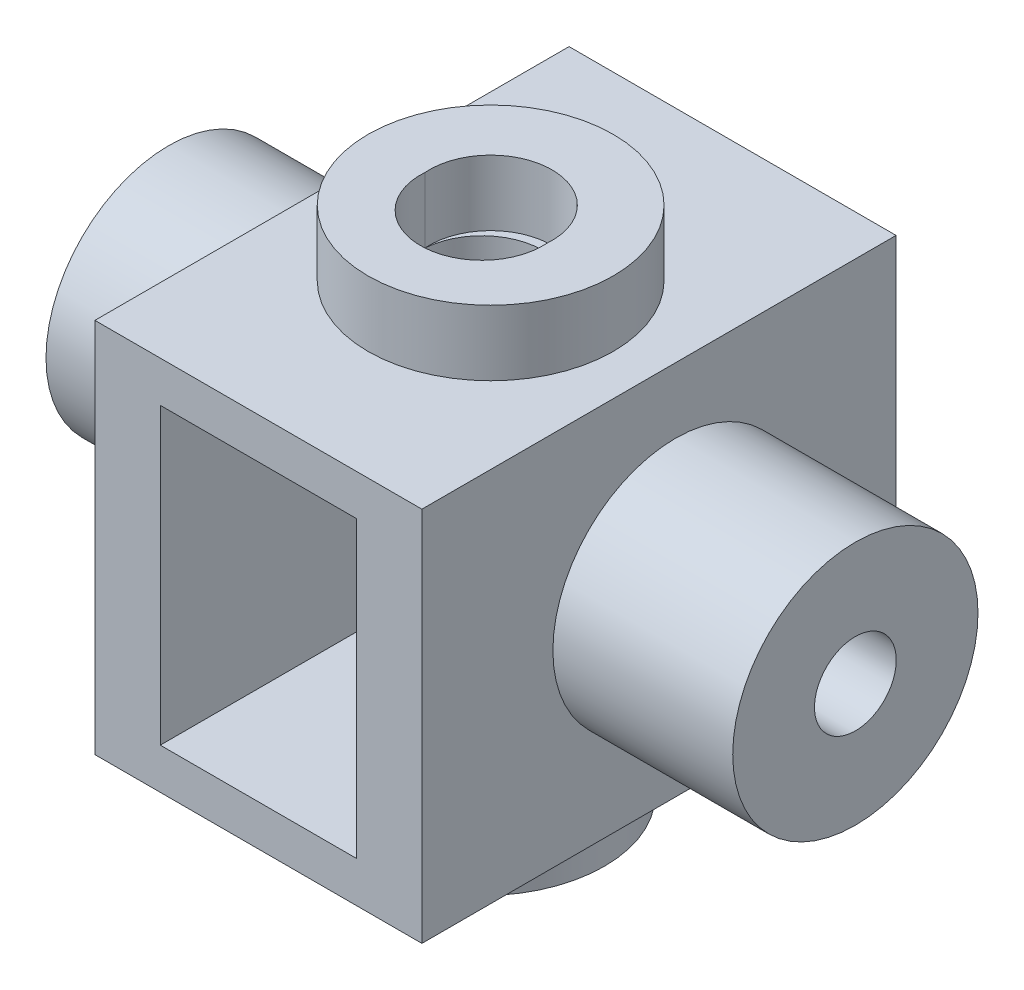
ISO-10303-21;
HEADER;
FILE_DESCRIPTION(('STEP AP214'),'2;1');
FILE_NAME('part.step','',(''),(''),'','','');
FILE_SCHEMA(('AUTOMOTIVE_DESIGN { 1 0 10303 214 1 1 1 1 }'));
ENDSEC;
DATA;
#1=APPLICATION_CONTEXT('core data for automotive mechanical design processes');
#2=APPLICATION_PROTOCOL_DEFINITION('international standard','automotive_design',2000,#1);
#3=PRODUCT_CONTEXT('',#1,'mechanical');
#4=PRODUCT('Part','Part','',(#3));
#5=PRODUCT_RELATED_PRODUCT_CATEGORY('part','',(#4));
#6=PRODUCT_DEFINITION_FORMATION('','',#4);
#7=PRODUCT_DEFINITION_CONTEXT('part definition',#1,'design');
#8=PRODUCT_DEFINITION('design','',#6,#7);
#9=PRODUCT_DEFINITION_SHAPE('','',#8);
#10=(LENGTH_UNIT() NAMED_UNIT(*) SI_UNIT(.MILLI.,.METRE.));
#11=(NAMED_UNIT(*) PLANE_ANGLE_UNIT() SI_UNIT($,.RADIAN.));
#12=(NAMED_UNIT(*) SI_UNIT($,.STERADIAN.) SOLID_ANGLE_UNIT());
#13=UNCERTAINTY_MEASURE_WITH_UNIT(LENGTH_MEASURE(1.E-05),#10,'distance_accuracy_value','');
#14=(GEOMETRIC_REPRESENTATION_CONTEXT(3) GLOBAL_UNCERTAINTY_ASSIGNED_CONTEXT((#13)) GLOBAL_UNIT_ASSIGNED_CONTEXT((#10,
#11,#12)) REPRESENTATION_CONTEXT('',''));
#15=CARTESIAN_POINT('',(0.,0.,0.));
#16=DIRECTION('',(0.,0.,1.));
#17=DIRECTION('',(1.,0.,0.));
#18=AXIS2_PLACEMENT_3D('',#15,#16,#17);
#19=CARTESIAN_POINT('',(-42.,23.,0.));
#20=DIRECTION('',(1.,0.,0.));
#21=DIRECTION('',(0.,0.,-1.));
#22=AXIS2_PLACEMENT_3D('',#19,#20,#21);
#23=PLANE('',#22);
#24=CARTESIAN_POINT('',(-42.,0.,-24.7911880329355));
#25=DIRECTION('',(1.,0.,0.));
#26=DIRECTION('',(0.,0.,-1.));
#27=AXIS2_PLACEMENT_3D('',#24,#25,#26);
#28=CIRCLE('',#27,5.);
#29=CARTESIAN_POINT('',(-42.,0.,-29.7911880329355));
#30=VERTEX_POINT('',#29);
#31=EDGE_CURVE('E146',#30,#30,#28,.T.);
#32=ORIENTED_EDGE('',*,*,#31,.T.);
#33=EDGE_LOOP('',(#32));
#34=FACE_BOUND('',#33,.T.);
#35=CARTESIAN_POINT('',(-42.,0.,-24.7911880329355));
#36=DIRECTION('',(-1.,0.,0.));
#37=DIRECTION('',(0.,0.,1.));
#38=AXIS2_PLACEMENT_3D('',#35,#36,#37);
#39=CIRCLE('',#38,15.);
#40=CARTESIAN_POINT('',(-42.,0.,-9.79118803293545));
#41=VERTEX_POINT('',#40);
#42=EDGE_CURVE('E258',#41,#41,#39,.T.);
#43=ORIENTED_EDGE('',*,*,#42,.T.);
#44=EDGE_LOOP('',(#43));
#45=FACE_BOUND('',#44,.T.);
#46=ADVANCED_FACE('F41',(#34,#45),#23,.F.);
#47=CARTESIAN_POINT('',(42.,23.,0.));
#48=DIRECTION('',(-1.,0.,0.));
#49=DIRECTION('',(0.,0.,1.));
#50=AXIS2_PLACEMENT_3D('',#47,#48,#49);
#51=PLANE('',#50);
#52=CARTESIAN_POINT('',(42.,0.,-24.7911880329355));
#53=DIRECTION('',(1.,0.,0.));
#54=DIRECTION('',(0.,0.,-1.));
#55=AXIS2_PLACEMENT_3D('',#52,#53,#54);
#56=CIRCLE('',#55,5.);
#57=CARTESIAN_POINT('',(42.,0.,-29.7911880329355));
#58=VERTEX_POINT('',#57);
#59=EDGE_CURVE('E143',#58,#58,#56,.T.);
#60=ORIENTED_EDGE('',*,*,#59,.F.);
#61=EDGE_LOOP('',(#60));
#62=FACE_BOUND('',#61,.T.);
#63=CARTESIAN_POINT('',(42.,0.,-24.7911880329355));
#64=DIRECTION('',(1.,0.,0.));
#65=DIRECTION('',(0.,0.,-1.));
#66=AXIS2_PLACEMENT_3D('',#63,#64,#65);
#67=CIRCLE('',#66,15.);
#68=CARTESIAN_POINT('',(42.,0.,-39.7911880329355));
#69=VERTEX_POINT('',#68);
#70=EDGE_CURVE('E157',#69,#69,#67,.T.);
#71=ORIENTED_EDGE('',*,*,#70,.T.);
#72=EDGE_LOOP('',(#71));
#73=FACE_BOUND('',#72,.T.);
#74=ADVANCED_FACE('F292',(#62,#73),#51,.F.);
#75=CARTESIAN_POINT('',(0.,23.,0.));
#76=DIRECTION('',(0.,1.,0.));
#77=DIRECTION('',(0.,0.,1.));
#78=AXIS2_PLACEMENT_3D('',#75,#76,#77);
#79=PLANE('',#78);
#80=DIRECTION('',(0.,0.,-1.));
#81=VECTOR('',#80,1.);
#82=CARTESIAN_POINT('',(-20.,23.,0.));
#83=LINE('',#82,#81);
#84=CARTESIAN_POINT('',(-20.,23.,6.23001766233769));
#85=VERTEX_POINT('',#84);
#86=CARTESIAN_POINT('',(-20.,23.,-51.7699823376623));
#87=VERTEX_POINT('',#86);
#88=EDGE_CURVE('E204',#85,#87,#83,.T.);
#89=ORIENTED_EDGE('',*,*,#88,.F.);
#90=DIRECTION('',(1.,0.,0.));
#91=VECTOR('',#90,1.);
#92=CARTESIAN_POINT('',(0.,23.,6.23001766233769));
#93=LINE('',#92,#91);
#94=CARTESIAN_POINT('',(20.,23.,6.23001766233769));
#95=VERTEX_POINT('',#94);
#96=EDGE_CURVE('E207',#85,#95,#93,.T.);
#97=ORIENTED_EDGE('',*,*,#96,.T.);
#98=DIRECTION('',(0.,0.,-1.));
#99=VECTOR('',#98,1.);
#100=CARTESIAN_POINT('',(20.,23.,0.));
#101=LINE('',#100,#99);
#102=CARTESIAN_POINT('',(20.,23.,-51.7699823376623));
#103=VERTEX_POINT('',#102);
#104=EDGE_CURVE('E200',#95,#103,#101,.T.);
#105=ORIENTED_EDGE('',*,*,#104,.T.);
#106=DIRECTION('',(1.,0.,0.));
#107=VECTOR('',#106,1.);
#108=CARTESIAN_POINT('',(0.,23.,-51.7699823376623));
#109=LINE('',#108,#107);
#110=EDGE_CURVE('E199',#87,#103,#109,.T.);
#111=ORIENTED_EDGE('',*,*,#110,.F.);
#112=EDGE_LOOP('',(#89,#97,#105,#111));
#113=FACE_BOUND('',#112,.T.);
#114=CARTESIAN_POINT('',(0.,23.,-22.1796347074505));
#115=DIRECTION('',(0.,1.,0.));
#116=DIRECTION('',(0.,0.,1.));
#117=AXIS2_PLACEMENT_3D('',#114,#115,#116);
#118=CIRCLE('',#117,15.);
#119=CARTESIAN_POINT('',(0.,23.,-7.17963470745051));
#120=VERTEX_POINT('',#119);
#121=EDGE_CURVE('E188',#120,#120,#118,.T.);
#122=ORIENTED_EDGE('',*,*,#121,.F.);
#123=EDGE_LOOP('',(#122));
#124=FACE_BOUND('',#123,.T.);
#125=ADVANCED_FACE('F237',(#113,#124),#79,.T.);
#126=CARTESIAN_POINT('',(0.,-23.,0.));
#127=DIRECTION('',(0.,1.,0.));
#128=DIRECTION('',(0.,0.,1.));
#129=AXIS2_PLACEMENT_3D('',#126,#127,#128);
#130=PLANE('',#129);
#131=CARTESIAN_POINT('',(0.,-23.,-21.0973307187279));
#132=DIRECTION('',(0.,1.,0.));
#133=DIRECTION('',(0.,0.,1.));
#134=AXIS2_PLACEMENT_3D('',#131,#132,#133);
#135=CIRCLE('',#134,15.);
#136=CARTESIAN_POINT('',(0.,-23.,-6.09733071872788));
#137=VERTEX_POINT('',#136);
#138=EDGE_CURVE('E11',#137,#137,#135,.F.);
#139=ORIENTED_EDGE('',*,*,#138,.F.);
#140=EDGE_LOOP('',(#139));
#141=FACE_BOUND('',#140,.T.);
#142=DIRECTION('',(0.,0.,1.));
#143=VECTOR('',#142,1.);
#144=CARTESIAN_POINT('',(-20.,-23.,0.));
#145=LINE('',#144,#143);
#146=CARTESIAN_POINT('',(-20.,-23.,-51.7699823376623));
#147=VERTEX_POINT('',#146);
#148=CARTESIAN_POINT('',(-20.,-23.,6.23001766233769));
#149=VERTEX_POINT('',#148);
#150=EDGE_CURVE('E215',#147,#149,#145,.T.);
#151=ORIENTED_EDGE('',*,*,#150,.F.);
#152=DIRECTION('',(1.,0.,0.));
#153=VECTOR('',#152,1.);
#154=CARTESIAN_POINT('',(0.,-23.,-51.7699823376623));
#155=LINE('',#154,#153);
#156=CARTESIAN_POINT('',(20.,-23.,-51.7699823376623));
#157=VERTEX_POINT('',#156);
#158=EDGE_CURVE('E191',#147,#157,#155,.T.);
#159=ORIENTED_EDGE('',*,*,#158,.T.);
#160=DIRECTION('',(0.,0.,1.));
#161=VECTOR('',#160,1.);
#162=CARTESIAN_POINT('',(20.,-23.,0.));
#163=LINE('',#162,#161);
#164=CARTESIAN_POINT('',(20.,-23.,6.23001766233769));
#165=VERTEX_POINT('',#164);
#166=EDGE_CURVE('E196',#157,#165,#163,.T.);
#167=ORIENTED_EDGE('',*,*,#166,.T.);
#168=DIRECTION('',(1.,0.,0.));
#169=VECTOR('',#168,1.);
#170=CARTESIAN_POINT('',(0.,-23.,6.23001766233769));
#171=LINE('',#170,#169);
#172=EDGE_CURVE('E211',#149,#165,#171,.T.);
#173=ORIENTED_EDGE('',*,*,#172,.F.);
#174=EDGE_LOOP('',(#151,#159,#167,#173));
#175=FACE_BOUND('',#174,.T.);
#176=ADVANCED_FACE('F235',(#141,#175),#130,.F.);
#177=CARTESIAN_POINT('',(0.,23.,-51.7699823376623));
#178=DIRECTION('',(0.,0.,-1.));
#179=DIRECTION('',(-1.,0.,0.));
#180=AXIS2_PLACEMENT_3D('',#177,#178,#179);
#181=PLANE('',#180);
#182=DIRECTION('',(0.,-1.,0.));
#183=VECTOR('',#182,1.);
#184=CARTESIAN_POINT('',(12.,23.,-51.7699823376623));
#185=LINE('',#184,#183);
#186=CARTESIAN_POINT('',(12.,18.,-51.7699823376623));
#187=VERTEX_POINT('',#186);
#188=CARTESIAN_POINT('',(12.,-18.,-51.7699823376623));
#189=VERTEX_POINT('',#188);
#190=EDGE_CURVE('E190',#187,#189,#185,.T.);
#191=ORIENTED_EDGE('',*,*,#190,.F.);
#192=DIRECTION('',(1.,0.,0.));
#193=VECTOR('',#192,1.);
#194=CARTESIAN_POINT('',(0.,18.,-51.7699823376623));
#195=LINE('',#194,#193);
#196=CARTESIAN_POINT('',(-12.,18.,-51.7699823376623));
#197=VERTEX_POINT('',#196);
#198=EDGE_CURVE('E176',#197,#187,#195,.T.);
#199=ORIENTED_EDGE('',*,*,#198,.F.);
#200=DIRECTION('',(0.,1.,0.));
#201=VECTOR('',#200,1.);
#202=CARTESIAN_POINT('',(-12.,23.,-51.7699823376623));
#203=LINE('',#202,#201);
#204=CARTESIAN_POINT('',(-12.,-18.,-51.7699823376623));
#205=VERTEX_POINT('',#204);
#206=EDGE_CURVE('E182',#205,#197,#203,.T.);
#207=ORIENTED_EDGE('',*,*,#206,.F.);
#208=DIRECTION('',(-1.,0.,0.));
#209=VECTOR('',#208,1.);
#210=CARTESIAN_POINT('',(0.,-18.,-51.7699823376623));
#211=LINE('',#210,#209);
#212=EDGE_CURVE('E184',#189,#205,#211,.T.);
#213=ORIENTED_EDGE('',*,*,#212,.F.);
#214=EDGE_LOOP('',(#191,#199,#207,#213));
#215=FACE_BOUND('',#214,.T.);
#216=ORIENTED_EDGE('',*,*,#158,.F.);
#217=DIRECTION('',(0.,-1.,0.));
#218=VECTOR('',#217,1.);
#219=CARTESIAN_POINT('',(-20.,23.,-51.7699823376623));
#220=LINE('',#219,#218);
#221=EDGE_CURVE('E139',#87,#147,#220,.T.);
#222=ORIENTED_EDGE('',*,*,#221,.F.);
#223=ORIENTED_EDGE('',*,*,#110,.T.);
#224=DIRECTION('',(0.,-1.,0.));
#225=VECTOR('',#224,1.);
#226=CARTESIAN_POINT('',(20.,23.,-51.7699823376623));
#227=LINE('',#226,#225);
#228=EDGE_CURVE('E131',#103,#157,#227,.T.);
#229=ORIENTED_EDGE('',*,*,#228,.T.);
#230=EDGE_LOOP('',(#216,#222,#223,#229));
#231=FACE_BOUND('',#230,.T.);
#232=ADVANCED_FACE('F43',(#215,#231),#181,.T.);
#233=CARTESIAN_POINT('',(-20.,23.,0.));
#234=DIRECTION('',(1.,0.,0.));
#235=DIRECTION('',(0.,0.,-1.));
#236=AXIS2_PLACEMENT_3D('',#233,#234,#235);
#237=PLANE('',#236);
#238=ORIENTED_EDGE('',*,*,#150,.T.);
#239=DIRECTION('',(0.,-1.,0.));
#240=VECTOR('',#239,1.);
#241=CARTESIAN_POINT('',(-20.,23.,6.23001766233769));
#242=LINE('',#241,#240);
#243=EDGE_CURVE('E216',#85,#149,#242,.T.);
#244=ORIENTED_EDGE('',*,*,#243,.F.);
#245=ORIENTED_EDGE('',*,*,#88,.T.);
#246=ORIENTED_EDGE('',*,*,#221,.T.);
#247=EDGE_LOOP('',(#238,#244,#245,#246));
#248=FACE_BOUND('',#247,.T.);
#249=CARTESIAN_POINT('',(-20.,0.,-24.7911880329355));
#250=DIRECTION('',(-1.,0.,0.));
#251=DIRECTION('',(0.,0.,1.));
#252=AXIS2_PLACEMENT_3D('',#249,#250,#251);
#253=CIRCLE('',#252,15.);
#254=CARTESIAN_POINT('',(-20.,0.,-9.79118803293545));
#255=VERTEX_POINT('',#254);
#256=EDGE_CURVE('E259',#255,#255,#253,.T.);
#257=ORIENTED_EDGE('',*,*,#256,.F.);
#258=EDGE_LOOP('',(#257));
#259=FACE_BOUND('',#258,.T.);
#260=ADVANCED_FACE('F225',(#248,#259),#237,.F.);
#261=CARTESIAN_POINT('',(0.,23.,6.23001766233769));
#262=DIRECTION('',(0.,0.,-1.));
#263=DIRECTION('',(-1.,0.,0.));
#264=AXIS2_PLACEMENT_3D('',#261,#262,#263);
#265=PLANE('',#264);
#266=DIRECTION('',(-1.,0.,0.));
#267=VECTOR('',#266,1.);
#268=CARTESIAN_POINT('',(-12.,18.,6.23001766233769));
#269=LINE('',#268,#267);
#270=CARTESIAN_POINT('',(12.,18.,6.23001766233769));
#271=VERTEX_POINT('',#270);
#272=CARTESIAN_POINT('',(-12.,18.,6.23001766233769));
#273=VERTEX_POINT('',#272);
#274=EDGE_CURVE('E164',#271,#273,#269,.T.);
#275=ORIENTED_EDGE('',*,*,#274,.F.);
#276=DIRECTION('',(0.,1.,0.));
#277=VECTOR('',#276,1.);
#278=CARTESIAN_POINT('',(12.,18.,6.23001766233769));
#279=LINE('',#278,#277);
#280=CARTESIAN_POINT('',(12.,-18.,6.23001766233769));
#281=VERTEX_POINT('',#280);
#282=EDGE_CURVE('E161',#281,#271,#279,.T.);
#283=ORIENTED_EDGE('',*,*,#282,.F.);
#284=DIRECTION('',(1.,0.,0.));
#285=VECTOR('',#284,1.);
#286=CARTESIAN_POINT('',(-12.,-18.,6.23001766233769));
#287=LINE('',#286,#285);
#288=CARTESIAN_POINT('',(-12.,-18.,6.23001766233769));
#289=VERTEX_POINT('',#288);
#290=EDGE_CURVE('E167',#289,#281,#287,.T.);
#291=ORIENTED_EDGE('',*,*,#290,.F.);
#292=DIRECTION('',(0.,-1.,0.));
#293=VECTOR('',#292,1.);
#294=CARTESIAN_POINT('',(-12.,18.,6.23001766233769));
#295=LINE('',#294,#293);
#296=EDGE_CURVE('E170',#273,#289,#295,.T.);
#297=ORIENTED_EDGE('',*,*,#296,.F.);
#298=EDGE_LOOP('',(#275,#283,#291,#297));
#299=FACE_BOUND('',#298,.T.);
#300=ORIENTED_EDGE('',*,*,#172,.T.);
#301=DIRECTION('',(0.,-1.,0.));
#302=VECTOR('',#301,1.);
#303=CARTESIAN_POINT('',(20.,23.,6.23001766233769));
#304=LINE('',#303,#302);
#305=EDGE_CURVE('E209',#95,#165,#304,.T.);
#306=ORIENTED_EDGE('',*,*,#305,.F.);
#307=ORIENTED_EDGE('',*,*,#96,.F.);
#308=ORIENTED_EDGE('',*,*,#243,.T.);
#309=EDGE_LOOP('',(#300,#306,#307,#308));
#310=FACE_BOUND('',#309,.T.);
#311=ADVANCED_FACE('F236',(#299,#310),#265,.F.);
#312=CARTESIAN_POINT('',(20.,23.,0.));
#313=DIRECTION('',(1.,0.,0.));
#314=DIRECTION('',(0.,0.,-1.));
#315=AXIS2_PLACEMENT_3D('',#312,#313,#314);
#316=PLANE('',#315);
#317=ORIENTED_EDGE('',*,*,#166,.F.);
#318=ORIENTED_EDGE('',*,*,#228,.F.);
#319=ORIENTED_EDGE('',*,*,#104,.F.);
#320=ORIENTED_EDGE('',*,*,#305,.T.);
#321=EDGE_LOOP('',(#317,#318,#319,#320));
#322=FACE_BOUND('',#321,.T.);
#323=CARTESIAN_POINT('',(20.,0.,-24.7911880329355));
#324=DIRECTION('',(1.,0.,0.));
#325=DIRECTION('',(0.,0.,-1.));
#326=AXIS2_PLACEMENT_3D('',#323,#324,#325);
#327=CIRCLE('',#326,15.);
#328=CARTESIAN_POINT('',(20.,0.,-39.7911880329355));
#329=VERTEX_POINT('',#328);
#330=EDGE_CURVE('E155',#329,#329,#327,.T.);
#331=ORIENTED_EDGE('',*,*,#330,.F.);
#332=EDGE_LOOP('',(#331));
#333=FACE_BOUND('',#332,.T.);
#334=ADVANCED_FACE('F245',(#322,#333),#316,.T.);
#335=CARTESIAN_POINT('',(0.,31.,-22.1796347074505));
#336=DIRECTION('',(0.,1.,0.));
#337=DIRECTION('',(0.,0.,1.));
#338=AXIS2_PLACEMENT_3D('',#335,#336,#337);
#339=PLANE('',#338);
#340=CARTESIAN_POINT('',(0.,31.,-21.0973307187279));
#341=DIRECTION('',(0.,1.,0.));
#342=DIRECTION('',(0.,0.,1.));
#343=AXIS2_PLACEMENT_3D('',#340,#341,#342);
#344=CIRCLE('',#343,7.5);
#345=CARTESIAN_POINT('',(-7.48045149165468,31.,-21.6384827130892));
#346=VERTEX_POINT('',#345);
#347=CARTESIAN_POINT('',(7.48045149165468,31.,-21.6384827130892));
#348=VERTEX_POINT('',#347);
#349=EDGE_CURVE('E135',#346,#348,#344,.T.);
#350=ORIENTED_EDGE('',*,*,#349,.F.);
#351=CARTESIAN_POINT('',(0.,31.,-22.1796347074505));
#352=DIRECTION('',(0.,1.,0.));
#353=DIRECTION('',(0.,0.,1.));
#354=AXIS2_PLACEMENT_3D('',#351,#352,#353);
#355=CIRCLE('',#354,7.5);
#356=EDGE_CURVE('E132',#348,#346,#355,.T.);
#357=ORIENTED_EDGE('',*,*,#356,.F.);
#358=EDGE_LOOP('',(#350,#357));
#359=FACE_BOUND('',#358,.T.);
#360=CARTESIAN_POINT('',(0.,31.,-22.1796347074505));
#361=DIRECTION('',(0.,1.,0.));
#362=DIRECTION('',(0.,0.,1.));
#363=AXIS2_PLACEMENT_3D('',#360,#361,#362);
#364=CIRCLE('',#363,15.);
#365=CARTESIAN_POINT('',(0.,31.,-7.17963470745051));
#366=VERTEX_POINT('',#365);
#367=EDGE_CURVE('E192',#366,#366,#364,.T.);
#368=ORIENTED_EDGE('',*,*,#367,.T.);
#369=EDGE_LOOP('',(#368));
#370=FACE_BOUND('',#369,.T.);
#371=ADVANCED_FACE('F244',(#359,#370),#339,.T.);
#372=CARTESIAN_POINT('',(0.,31.,-22.1796347074505));
#373=DIRECTION('',(0.,-1.,0.));
#374=DIRECTION('',(0.,0.,-1.));
#375=AXIS2_PLACEMENT_3D('',#372,#373,#374);
#376=CYLINDRICAL_SURFACE('',#375,15.);
#377=ORIENTED_EDGE('',*,*,#367,.F.);
#378=EDGE_LOOP('',(#377));
#379=FACE_BOUND('',#378,.T.);
#380=ORIENTED_EDGE('',*,*,#121,.T.);
#381=EDGE_LOOP('',(#380));
#382=FACE_BOUND('',#381,.T.);
#383=ADVANCED_FACE('F311',(#379,#382),#376,.T.);
#384=CARTESIAN_POINT('',(0.,31.,-22.1796347074505));
#385=DIRECTION('',(0.,-1.,0.));
#386=DIRECTION('',(0.,0.,-1.));
#387=AXIS2_PLACEMENT_3D('',#384,#385,#386);
#388=CYLINDRICAL_SURFACE('',#387,7.5);
#389=DIRECTION('',(0.,-1.,0.));
#390=VECTOR('',#389,1.);
#391=CARTESIAN_POINT('',(-7.48045149165468,7.50000000000001,-21.6384827130892));
#392=LINE('',#391,#390);
#393=CARTESIAN_POINT('',(-7.48045149165468,23.,-21.6384827130892));
#394=VERTEX_POINT('',#393);
#395=EDGE_CURVE('E119',#394,#346,#392,.F.);
#396=ORIENTED_EDGE('',*,*,#395,.F.);
#397=CARTESIAN_POINT('',(0.,23.,-22.1796347074505));
#398=DIRECTION('',(0.,1.,0.));
#399=DIRECTION('',(0.,0.,1.));
#400=AXIS2_PLACEMENT_3D('',#397,#398,#399);
#401=CIRCLE('',#400,7.5);
#402=CARTESIAN_POINT('',(7.48045149165468,23.,-21.6384827130892));
#403=VERTEX_POINT('',#402);
#404=EDGE_CURVE('E49',#394,#403,#401,.F.);
#405=ORIENTED_EDGE('',*,*,#404,.T.);
#406=DIRECTION('',(0.,-1.,0.));
#407=VECTOR('',#406,1.);
#408=CARTESIAN_POINT('',(7.48045149165468,7.50000000000001,-21.6384827130892));
#409=LINE('',#408,#407);
#410=EDGE_CURVE('E60',#348,#403,#409,.T.);
#411=ORIENTED_EDGE('',*,*,#410,.F.);
#412=ORIENTED_EDGE('',*,*,#356,.T.);
#413=EDGE_LOOP('',(#396,#405,#411,#412));
#414=FACE_BOUND('',#413,.T.);
#415=ADVANCED_FACE('F126',(#414),#388,.F.);
#416=CARTESIAN_POINT('',(0.,23.,-21.0973307187279));
#417=DIRECTION('',(0.,1.,0.));
#418=DIRECTION('',(0.,0.,1.));
#419=AXIS2_PLACEMENT_3D('',#416,#417,#418);
#420=CIRCLE('',#419,7.5);
#421=EDGE_CURVE('E116',#403,#394,#420,.T.);
#422=ORIENTED_EDGE('',*,*,#421,.F.);
#423=ORIENTED_EDGE('',*,*,#404,.F.);
#424=EDGE_LOOP('',(#422,#423));
#425=FACE_BOUND('',#424,.T.);
#426=ADVANCED_FACE('F134',(#425),#79,.T.);
#427=CARTESIAN_POINT('',(12.,18.,-53.7699823376623));
#428=DIRECTION('',(1.,0.,0.));
#429=DIRECTION('',(0.,1.,0.));
#430=AXIS2_PLACEMENT_3D('',#427,#428,#429);
#431=PLANE('',#430);
#432=CARTESIAN_POINT('',(12.,0.,-24.7911880329355));
#433=DIRECTION('',(1.,0.,0.));
#434=DIRECTION('',(0.,1.,0.));
#435=AXIS2_PLACEMENT_3D('',#432,#433,#434);
#436=CIRCLE('',#435,5.);
#437=CARTESIAN_POINT('',(12.,5.,-24.7911880329355));
#438=VERTEX_POINT('',#437);
#439=EDGE_CURVE('E144',#438,#438,#436,.T.);
#440=ORIENTED_EDGE('',*,*,#439,.T.);
#441=EDGE_LOOP('',(#440));
#442=FACE_BOUND('',#441,.T.);
#443=ORIENTED_EDGE('',*,*,#190,.T.);
#444=DIRECTION('',(0.,0.,1.));
#445=VECTOR('',#444,1.);
#446=CARTESIAN_POINT('',(12.,-18.,-53.7699823376623));
#447=LINE('',#446,#445);
#448=EDGE_CURVE('E172',#189,#281,#447,.T.);
#449=ORIENTED_EDGE('',*,*,#448,.T.);
#450=ORIENTED_EDGE('',*,*,#282,.T.);
#451=DIRECTION('',(0.,0.,1.));
#452=VECTOR('',#451,1.);
#453=CARTESIAN_POINT('',(12.,18.,-53.7699823376623));
#454=LINE('',#453,#452);
#455=EDGE_CURVE('E173',#187,#271,#454,.T.);
#456=ORIENTED_EDGE('',*,*,#455,.F.);
#457=EDGE_LOOP('',(#443,#449,#450,#456));
#458=FACE_BOUND('',#457,.T.);
#459=ADVANCED_FACE('F318',(#442,#458),#431,.F.);
#460=CARTESIAN_POINT('',(-12.,-18.,-53.7699823376623));
#461=DIRECTION('',(0.,-1.,0.));
#462=DIRECTION('',(0.,0.,-1.));
#463=AXIS2_PLACEMENT_3D('',#460,#461,#462);
#464=PLANE('',#463);
#465=CARTESIAN_POINT('',(0.,-18.,-21.0973307187279));
#466=DIRECTION('',(0.,-1.,0.));
#467=DIRECTION('',(0.,0.,-1.));
#468=AXIS2_PLACEMENT_3D('',#465,#466,#467);
#469=CIRCLE('',#468,7.5);
#470=CARTESIAN_POINT('',(0.,-18.,-28.5973307187279));
#471=VERTEX_POINT('',#470);
#472=EDGE_CURVE('E123',#471,#471,#469,.T.);
#473=ORIENTED_EDGE('',*,*,#472,.T.);
#474=EDGE_LOOP('',(#473));
#475=FACE_BOUND('',#474,.T.);
#476=ORIENTED_EDGE('',*,*,#212,.T.);
#477=DIRECTION('',(0.,0.,1.));
#478=VECTOR('',#477,1.);
#479=CARTESIAN_POINT('',(-12.,-18.,-53.7699823376623));
#480=LINE('',#479,#478);
#481=EDGE_CURVE('E180',#205,#289,#480,.T.);
#482=ORIENTED_EDGE('',*,*,#481,.T.);
#483=ORIENTED_EDGE('',*,*,#290,.T.);
#484=ORIENTED_EDGE('',*,*,#448,.F.);
#485=EDGE_LOOP('',(#476,#482,#483,#484));
#486=FACE_BOUND('',#485,.T.);
#487=ADVANCED_FACE('F324',(#475,#486),#464,.F.);
#488=CARTESIAN_POINT('',(-12.,18.,-53.7699823376623));
#489=DIRECTION('',(-1.,0.,0.));
#490=DIRECTION('',(0.,-1.,0.));
#491=AXIS2_PLACEMENT_3D('',#488,#489,#490);
#492=PLANE('',#491);
#493=CARTESIAN_POINT('',(-12.,0.,-24.7911880329355));
#494=DIRECTION('',(-1.,0.,0.));
#495=DIRECTION('',(0.,-1.,0.));
#496=AXIS2_PLACEMENT_3D('',#493,#494,#495);
#497=CIRCLE('',#496,5.);
#498=CARTESIAN_POINT('',(-12.,-5.,-24.7911880329355));
#499=VERTEX_POINT('',#498);
#500=EDGE_CURVE('E145',#499,#499,#497,.T.);
#501=ORIENTED_EDGE('',*,*,#500,.T.);
#502=EDGE_LOOP('',(#501));
#503=FACE_BOUND('',#502,.T.);
#504=ORIENTED_EDGE('',*,*,#206,.T.);
#505=DIRECTION('',(0.,0.,1.));
#506=VECTOR('',#505,1.);
#507=CARTESIAN_POINT('',(-12.,18.,-53.7699823376623));
#508=LINE('',#507,#506);
#509=EDGE_CURVE('E63',#197,#273,#508,.T.);
#510=ORIENTED_EDGE('',*,*,#509,.T.);
#511=ORIENTED_EDGE('',*,*,#296,.T.);
#512=ORIENTED_EDGE('',*,*,#481,.F.);
#513=EDGE_LOOP('',(#504,#510,#511,#512));
#514=FACE_BOUND('',#513,.T.);
#515=ADVANCED_FACE('F328',(#503,#514),#492,.F.);
#516=CARTESIAN_POINT('',(-12.,18.,-53.7699823376623));
#517=DIRECTION('',(0.,1.,0.));
#518=DIRECTION('',(0.,0.,1.));
#519=AXIS2_PLACEMENT_3D('',#516,#517,#518);
#520=PLANE('',#519);
#521=CARTESIAN_POINT('',(0.,18.,-21.0973307187279));
#522=DIRECTION('',(0.,1.,0.));
#523=DIRECTION('',(0.,0.,1.));
#524=AXIS2_PLACEMENT_3D('',#521,#522,#523);
#525=CIRCLE('',#524,7.5);
#526=CARTESIAN_POINT('',(0.,18.,-13.5973307187279));
#527=VERTEX_POINT('',#526);
#528=EDGE_CURVE('E44',#527,#527,#525,.T.);
#529=ORIENTED_EDGE('',*,*,#528,.T.);
#530=EDGE_LOOP('',(#529));
#531=FACE_BOUND('',#530,.T.);
#532=ORIENTED_EDGE('',*,*,#198,.T.);
#533=ORIENTED_EDGE('',*,*,#455,.T.);
#534=ORIENTED_EDGE('',*,*,#274,.T.);
#535=ORIENTED_EDGE('',*,*,#509,.F.);
#536=EDGE_LOOP('',(#532,#533,#534,#535));
#537=FACE_BOUND('',#536,.T.);
#538=ADVANCED_FACE('F282',(#531,#537),#520,.F.);
#539=CARTESIAN_POINT('',(-53.,0.,-24.7911880329355));
#540=DIRECTION('',(1.,0.,0.));
#541=DIRECTION('',(0.,0.,-1.));
#542=AXIS2_PLACEMENT_3D('',#539,#540,#541);
#543=CYLINDRICAL_SURFACE('',#542,5.);
#544=ORIENTED_EDGE('',*,*,#500,.F.);
#545=EDGE_LOOP('',(#544));
#546=FACE_BOUND('',#545,.T.);
#547=ORIENTED_EDGE('',*,*,#31,.F.);
#548=EDGE_LOOP('',(#547));
#549=FACE_BOUND('',#548,.T.);
#550=ADVANCED_FACE('F330',(#546,#549),#543,.F.);
#551=ORIENTED_EDGE('',*,*,#59,.T.);
#552=EDGE_LOOP('',(#551));
#553=FACE_BOUND('',#552,.T.);
#554=ORIENTED_EDGE('',*,*,#439,.F.);
#555=EDGE_LOOP('',(#554));
#556=FACE_BOUND('',#555,.T.);
#557=ADVANCED_FACE('F254',(#553,#556),#543,.F.);
#558=CARTESIAN_POINT('',(20.,0.,-24.7911880329355));
#559=DIRECTION('',(1.,0.,0.));
#560=DIRECTION('',(0.,0.,-1.));
#561=AXIS2_PLACEMENT_3D('',#558,#559,#560);
#562=CYLINDRICAL_SURFACE('',#561,15.);
#563=ORIENTED_EDGE('',*,*,#330,.T.);
#564=EDGE_LOOP('',(#563));
#565=FACE_BOUND('',#564,.T.);
#566=ORIENTED_EDGE('',*,*,#70,.F.);
#567=EDGE_LOOP('',(#566));
#568=FACE_BOUND('',#567,.T.);
#569=ADVANCED_FACE('F248',(#565,#568),#562,.T.);
#570=CARTESIAN_POINT('',(-20.,0.,-24.7911880329355));
#571=DIRECTION('',(-1.,0.,0.));
#572=DIRECTION('',(0.,0.,1.));
#573=AXIS2_PLACEMENT_3D('',#570,#571,#572);
#574=CYLINDRICAL_SURFACE('',#573,15.);
#575=ORIENTED_EDGE('',*,*,#256,.T.);
#576=EDGE_LOOP('',(#575));
#577=FACE_BOUND('',#576,.T.);
#578=ORIENTED_EDGE('',*,*,#42,.F.);
#579=EDGE_LOOP('',(#578));
#580=FACE_BOUND('',#579,.T.);
#581=ADVANCED_FACE('F255',(#577,#580),#574,.T.);
#582=CARTESIAN_POINT('',(0.,-31.,-21.0973307187279));
#583=DIRECTION('',(0.,-1.,0.));
#584=DIRECTION('',(0.,0.,-1.));
#585=AXIS2_PLACEMENT_3D('',#582,#583,#584);
#586=PLANE('',#585);
#587=CARTESIAN_POINT('',(0.,-31.,-21.0973307187279));
#588=DIRECTION('',(0.,-1.,0.));
#589=DIRECTION('',(0.,0.,-1.));
#590=AXIS2_PLACEMENT_3D('',#587,#588,#589);
#591=CIRCLE('',#590,15.);
#592=CARTESIAN_POINT('',(0.,-31.,-36.0973307187279));
#593=VERTEX_POINT('',#592);
#594=EDGE_CURVE('E261',#593,#593,#591,.T.);
#595=ORIENTED_EDGE('',*,*,#594,.T.);
#596=EDGE_LOOP('',(#595));
#597=FACE_BOUND('',#596,.T.);
#598=CARTESIAN_POINT('',(0.,-31.,-21.0973307187279));
#599=DIRECTION('',(0.,-1.,0.));
#600=DIRECTION('',(0.,0.,-1.));
#601=AXIS2_PLACEMENT_3D('',#598,#599,#600);
#602=CIRCLE('',#601,7.5);
#603=CARTESIAN_POINT('',(0.,-31.,-28.5973307187279));
#604=VERTEX_POINT('',#603);
#605=EDGE_CURVE('E270',#604,#604,#602,.T.);
#606=ORIENTED_EDGE('',*,*,#605,.F.);
#607=EDGE_LOOP('',(#606));
#608=FACE_BOUND('',#607,.T.);
#609=ADVANCED_FACE('F336',(#597,#608),#586,.T.);
#610=CARTESIAN_POINT('',(0.,-31.,-21.0973307187279));
#611=DIRECTION('',(0.,1.,0.));
#612=DIRECTION('',(0.,0.,1.));
#613=AXIS2_PLACEMENT_3D('',#610,#611,#612);
#614=CYLINDRICAL_SURFACE('',#613,15.);
#615=ORIENTED_EDGE('',*,*,#594,.F.);
#616=EDGE_LOOP('',(#615));
#617=FACE_BOUND('',#616,.T.);
#618=ORIENTED_EDGE('',*,*,#138,.T.);
#619=EDGE_LOOP('',(#618));
#620=FACE_BOUND('',#619,.T.);
#621=ADVANCED_FACE('F289',(#617,#620),#614,.T.);
#622=CARTESIAN_POINT('',(0.,-31.,-21.0973307187279));
#623=DIRECTION('',(0.,1.,0.));
#624=DIRECTION('',(0.,0.,1.));
#625=AXIS2_PLACEMENT_3D('',#622,#623,#624);
#626=CYLINDRICAL_SURFACE('',#625,7.5);
#627=ORIENTED_EDGE('',*,*,#605,.T.);
#628=EDGE_LOOP('',(#627));
#629=FACE_BOUND('',#628,.T.);
#630=ORIENTED_EDGE('',*,*,#472,.F.);
#631=EDGE_LOOP('',(#630));
#632=FACE_BOUND('',#631,.T.);
#633=ADVANCED_FACE('F283',(#629,#632),#626,.F.);
#634=CARTESIAN_POINT('',(0.,38.,-21.0973307187279));
#635=DIRECTION('',(0.,-1.,0.));
#636=DIRECTION('',(0.,0.,-1.));
#637=AXIS2_PLACEMENT_3D('',#634,#635,#636);
#638=CYLINDRICAL_SURFACE('',#637,7.5);
#639=ORIENTED_EDGE('',*,*,#349,.T.);
#640=ORIENTED_EDGE('',*,*,#410,.T.);
#641=ORIENTED_EDGE('',*,*,#421,.T.);
#642=ORIENTED_EDGE('',*,*,#395,.T.);
#643=EDGE_LOOP('',(#639,#640,#641,#642));
#644=FACE_BOUND('',#643,.T.);
#645=ORIENTED_EDGE('',*,*,#528,.F.);
#646=EDGE_LOOP('',(#645));
#647=FACE_BOUND('',#646,.T.);
#648=ADVANCED_FACE('F117',(#644,#647),#638,.F.);
#649=CLOSED_SHELL('',(#46,#74,#125,#176,#232,#260,#311,#334,#371,#383,#415,#426,#459,#487,#515,
#538,#550,#557,#569,#581,#609,#621,#633,#648));
#650=MANIFOLD_SOLID_BREP('B2',#649);
#651=ADVANCED_BREP_SHAPE_REPRESENTATION('',(#18,#650),#14);
#652=SHAPE_DEFINITION_REPRESENTATION(#9,#651);
ENDSEC;
END-ISO-10303-21;
